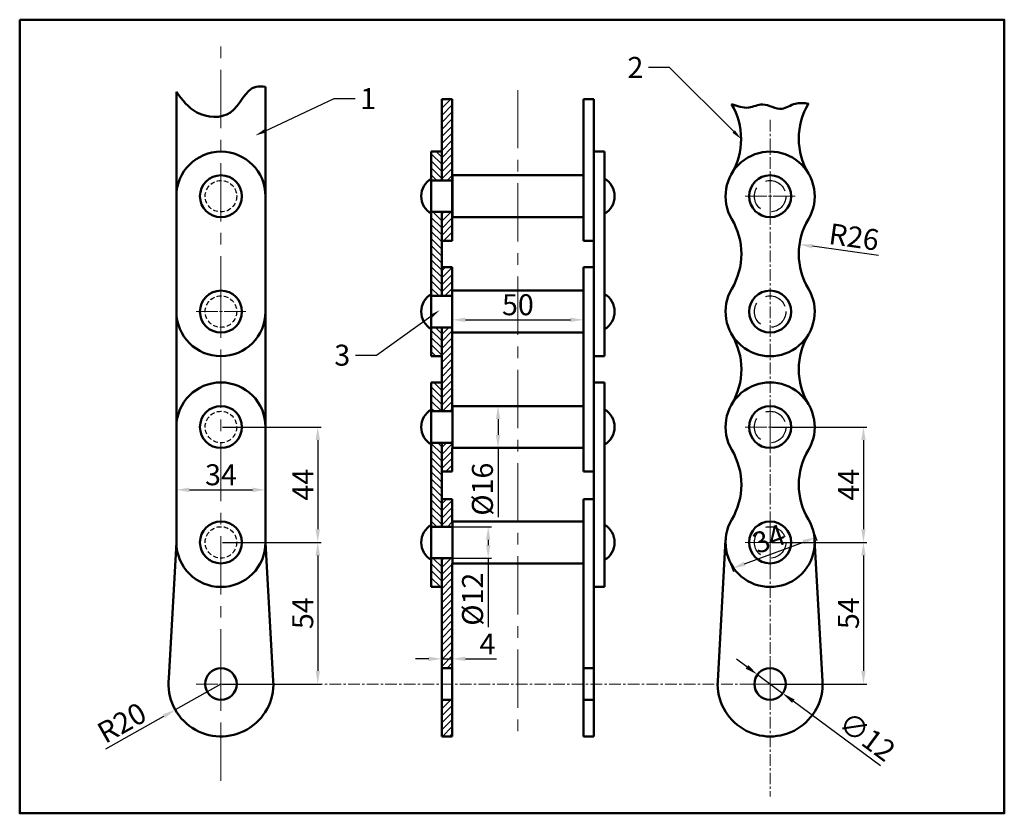
# Model space of a CAD drawing. Units: millimetres. Extents: x 359 to 734, y 213 to 516.
import ezdxf
from ezdxf import colors
from ezdxf.entities.mleader import LeaderData, LeaderLine
from ezdxf.math import Vec2, Vec3

# ---------------------------------------------------------------- set-up
doc = ezdxf.new("R2010")
doc.units = ezdxf.units.MM
doc.header["$LTSCALE"] = 0.7
doc.linetypes.add('CENTER', pattern=[50.8, 31.75, -6.35, 6.35, -6.35])
doc.linetypes.add('DASHED', pattern=[19.05, 12.7, -6.35])
for name, color, linetype, lineweight in [('M-CNTR', 1, 'CENTER', 18), ('M-DIMS', 2, 'Continuous', 25), ('M-HATC', 8, 'Continuous', 18), ('M-HIDN', 6, 'DASHED', 25), ('M-OUTL', 7, 'Continuous', 50), ('M-TTLB', 7, 'Continuous', 50)]:
    doc.layers.add(name, color=color, linetype=linetype, lineweight=lineweight)
doc.styles.get("Standard").update_dxf_attribs({"font": 'arial.ttf'})
doc.dimstyles.new('ISO-25', dxfattribs={"dimtxt": 8, "dimasz": 5, "dimexe": 1.25, "dimexo": 0.625, "dimtad": 1, "dimdec": 0, "dimtxsty": 'Standard', "dimcen": 2.5, "dimadec": 0, "dimazin": 0, "dimtfac": 1, "dimtdec": 0, "dimtmove": 0, "dimatfit": 3, "dimfxl": 1, "dimarcsym": 0})

# ---------------------------------------------------------------- blocks, each defined once
blk = doc.blocks.new('*U1')
at = {"layer": 'M-CNTR', "color": 0, "transparency": 16777216}
for p, q in [((0, 1.2), (0, 9.5)), ((-9.5, 0), (-1.2, 0)), ((1.2, 0), (9.5, 0)), ((0, -9.5), (0, -1.2))]:
    blk.add_line(p, q, dxfattribs=at)
at = {"layer": 'M-CNTR', "color": 0, "linetype": 'Continuous', "transparency": 16777216}
for p, q in [((-0.6, 0), (0.6, 0)), ((0, -0.6), (0, 0.6))]:
    blk.add_line(p, q, dxfattribs=at)
blk = doc.blocks.new('*U2')
at = {"layer": 'M-CNTR', "color": 0, "transparency": 16777216}
for p, q in [((0, 1.2), (0, 9.5)), ((-9.5, 0), (-1.2, 0)), ((1.2, 0), (9.5, 0)), ((0, -9.5), (0, -1.2))]:
    blk.add_line(p, q, dxfattribs=at)
at = {"layer": 'M-CNTR', "color": 0, "linetype": 'Continuous', "transparency": 16777216}
for p, q in [((-0.6, 0), (0.6, 0)), ((0, -0.6), (0, 0.6))]:
    blk.add_line(p, q, dxfattribs=at)
blk = doc.blocks.new('*U3')
at = {"layer": 'M-CNTR', "color": 0, "transparency": 16777216}
for p, q in [((0, 1.2), (0, 9.5)), ((-9.5, 0), (-1.2, 0)), ((1.2, 0), (9.5, 0)), ((0, -9.5), (0, -1.2))]:
    blk.add_line(p, q, dxfattribs=at)
at = {"layer": 'M-CNTR', "color": 0, "linetype": 'Continuous', "transparency": 16777216}
for p, q in [((-0.6, 0), (0.6, 0)), ((0, -0.6), (0, 0.6))]:
    blk.add_line(p, q, dxfattribs=at)
blk = doc.blocks.new('*U4')
at = {"layer": 'M-CNTR', "color": 0, "transparency": 16777216}
for p, q in [((0, 1.2), (0, 9.5)), ((-9.5, 0), (-1.2, 0)), ((1.2, 0), (9.5, 0)), ((0, -9.5), (0, -1.2))]:
    blk.add_line(p, q, dxfattribs=at)
at = {"layer": 'M-CNTR', "color": 0, "linetype": 'Continuous', "transparency": 16777216}
for p, q in [((-0.6, 0), (0.6, 0)), ((0, -0.6), (0, 0.6))]:
    blk.add_line(p, q, dxfattribs=at)
blk = doc.blocks.new('*U5')
at = {"layer": 'M-CNTR', "color": 0, "transparency": 16777216}
for p, q in [((0, 1.2), (0, 9.5)), ((-9.5, 0), (-1.2, 0)), ((1.2, 0), (9.5, 0)), ((0, -9.5), (0, -1.2))]:
    blk.add_line(p, q, dxfattribs=at)
at = {"layer": 'M-CNTR', "color": 0, "linetype": 'Continuous', "transparency": 16777216}
for p, q in [((-0.6, 0), (0.6, 0)), ((0, -0.6), (0, 0.6))]:
    blk.add_line(p, q, dxfattribs=at)
blk = doc.blocks.new('*U6')
at = {"layer": 'M-CNTR', "color": 0, "transparency": 16777216}
for p, q in [((0, 1.2), (0, 9.5)), ((-9.5, 0), (-1.2, 0)), ((1.2, 0), (9.5, 0)), ((0, -9.5), (0, -1.2))]:
    blk.add_line(p, q, dxfattribs=at)
at = {"layer": 'M-CNTR', "color": 0, "linetype": 'Continuous', "transparency": 16777216}
for p, q in [((-0.6, 0), (0.6, 0)), ((0, -0.6), (0, 0.6))]:
    blk.add_line(p, q, dxfattribs=at)
blk = doc.blocks.new('*U7')
at = {"layer": 'M-CNTR', "color": 0, "transparency": 16777216}
blk.add_line((0, 18), (0, -229.67), dxfattribs=at)
blk = doc.blocks.new('*U8')
at = {"layer": 'M-CNTR', "color": 0, "transparency": 16777216}
blk.add_line((0, -156.93), (0, 123.49), dxfattribs=at)
blk = doc.blocks.new('*D9')
at = {"layer": 'Defpoints', "color": 0, "ltscale": 0.7, "transparency": 16777216}
for p in [(418.66, 336.41), (452.66, 336.64), (452.66, 336.41)]:
    blk.add_point(p, dxfattribs=at)
at = {"layer": 'M-DIMS', "color": 0, "lineweight": -2, "ltscale": 0.7, "transparency": 16777216}
for p, q in [((418.66, 337.04), (418.66, 337.89)), ((452.66, 337.04), (452.66, 337.89)), ((423.66, 336.64), (447.66, 336.64))]:
    blk.add_line(p, q, dxfattribs=at)
at = {"layer": 'M-DIMS', "color": 0, "ltscale": 0.7, "transparency": 16777216}
for points in [[(423.66, 337.48), (423.66, 335.81), (418.66, 336.64)], [(447.66, 337.48), (447.66, 335.81), (452.66, 336.64)]]:
    blk.add_solid(points, dxfattribs=at)
at = {"layer": 'M-DIMS', "color": 0, "ltscale": 0.7, "transparency": 16777216, "insert": (435.66, 341.35), "char_height": 8, "attachment_point": 5}
blk.add_mtext('34', dxfattribs=at)
blk = doc.blocks.new('*D10')
at = {"layer": 'Defpoints', "color": 0, "ltscale": 0.7, "transparency": 16777216}
for p in [(435.66, 360.6), (435.66, 316.6), (472.57, 316.6)]:
    blk.add_point(p, dxfattribs=at)
at = {"layer": 'M-DIMS', "color": 0, "lineweight": -2, "ltscale": 0.7, "transparency": 16777216}
for p, q in [((436.28, 360.6), (473.82, 360.6)), ((472.57, 355.6), (472.57, 321.6)), ((436.28, 316.6), (473.82, 316.6))]:
    blk.add_line(p, q, dxfattribs=at)
at = {"layer": 'M-DIMS', "color": 0, "ltscale": 0.7, "transparency": 16777216}
for points in [[(471.73, 355.6), (473.4, 355.6), (472.57, 360.6)], [(471.73, 321.6), (473.4, 321.6), (472.57, 316.6)]]:
    blk.add_solid(points, dxfattribs=at)
at = {"layer": 'M-DIMS', "color": 0, "ltscale": 0.7, "transparency": 16777216, "insert": (467.94, 338.6), "char_height": 8, "attachment_point": 5, "rotation": 90}
blk.add_mtext('44', dxfattribs=at)
blk = doc.blocks.new('*D11')
at = {"layer": 'Defpoints', "color": 0, "ltscale": 0.7, "transparency": 16777216}
for p in [(463.42, 316.6), (435.66, 262.6), (472.57, 262.6)]:
    blk.add_point(p, dxfattribs=at)
at = {"layer": 'M-DIMS', "color": 0, "lineweight": -2, "ltscale": 0.7, "transparency": 16777216}
for p, q in [((464.04, 316.6), (473.82, 316.6)), ((472.57, 311.6), (472.57, 267.6)), ((436.28, 262.6), (473.82, 262.6))]:
    blk.add_line(p, q, dxfattribs=at)
at = {"layer": 'M-DIMS', "color": 0, "ltscale": 0.7, "transparency": 16777216}
for points in [[(471.73, 311.6), (473.4, 311.6), (472.57, 316.6)], [(471.73, 267.6), (473.4, 267.6), (472.57, 262.6)]]:
    blk.add_solid(points, dxfattribs=at)
at = {"layer": 'M-DIMS', "color": 0, "ltscale": 0.7, "transparency": 16777216, "insert": (467.87, 289.6), "char_height": 8, "attachment_point": 5, "rotation": 90}
blk.add_mtext('54', dxfattribs=at)
blk = doc.blocks.new('*D12')
at = {"layer": 'Defpoints', "color": 0, "ltscale": 0.7, "transparency": 16777216}
for p in [(523.86, 404.6), (573.86, 404.6), (573.86, 401.48)]:
    blk.add_point(p, dxfattribs=at)
at = {"layer": 'M-DIMS', "color": 0, "lineweight": -2, "ltscale": 0.7, "transparency": 16777216}
for p, q in [((523.86, 403.97), (523.86, 400.23)), ((573.86, 403.97), (573.86, 400.23)), ((528.86, 401.48), (568.86, 401.48))]:
    blk.add_line(p, q, dxfattribs=at)
at = {"layer": 'M-DIMS', "color": 0, "ltscale": 0.7, "transparency": 16777216}
for points in [[(528.86, 402.31), (528.86, 400.65), (523.86, 401.48)], [(568.86, 402.31), (568.86, 400.65), (573.86, 401.48)]]:
    blk.add_solid(points, dxfattribs=at)
at = {"layer": 'M-DIMS', "color": 0, "ltscale": 0.7, "transparency": 16777216, "insert": (548.86, 406.19), "char_height": 8, "attachment_point": 5}
blk.add_mtext('50', dxfattribs=at)
blk = doc.blocks.new('*D13')
at = {"layer": 'Defpoints', "color": 0, "ltscale": 0.7, "transparency": 16777216}
for p in [(541.3, 368.6), (541.3, 352.6), (541.3, 352.6)]:
    blk.add_point(p, dxfattribs=at)
at = {"layer": 'M-DIMS', "color": 0, "lineweight": -2, "ltscale": 0.7, "transparency": 16777216}
for p, q in [((541.93, 368.6), (542.55, 368.6)), ((541.3, 363.6), (541.3, 357.6)), ((541.3, 352.6), (541.3, 326.19)), ((541.93, 352.6), (542.55, 352.6))]:
    blk.add_line(p, q, dxfattribs=at)
at = {"layer": 'M-DIMS', "color": 0, "ltscale": 0.7, "transparency": 16777216}
for points in [[(540.47, 363.6), (542.13, 363.6), (541.3, 368.6)], [(540.47, 357.6), (542.13, 357.6), (541.3, 352.6)]]:
    blk.add_solid(points, dxfattribs=at)
at = {"layer": 'M-DIMS', "color": 0, "ltscale": 0.7, "transparency": 16777216, "insert": (536.37, 336.89), "char_height": 8, "attachment_point": 5, "rotation": 90}
blk.add_mtext('%%C16', dxfattribs=at)
blk = doc.blocks.new('*D14')
at = {"layer": 'Defpoints', "color": 0, "ltscale": 0.7, "transparency": 16777216}
for p in [(523.86, 322.6), (523.86, 310.6), (537.54, 310.6)]:
    blk.add_point(p, dxfattribs=at)
at = {"layer": 'M-DIMS', "color": 0, "lineweight": -2, "ltscale": 0.7, "transparency": 16777216}
for p, q in [((524.49, 322.6), (538.79, 322.6)), ((537.54, 317.6), (537.54, 315.6)), ((524.49, 310.6), (538.79, 310.6)), ((537.54, 310.6), (537.54, 284.26))]:
    blk.add_line(p, q, dxfattribs=at)
at = {"layer": 'M-DIMS', "color": 0, "ltscale": 0.7, "transparency": 16777216}
for points in [[(536.7, 317.6), (538.37, 317.6), (537.54, 322.6)], [(536.7, 315.6), (538.37, 315.6), (537.54, 310.6)]]:
    blk.add_solid(points, dxfattribs=at)
at = {"layer": 'M-DIMS', "color": 0, "ltscale": 0.7, "transparency": 16777216, "insert": (532.6, 294.93), "char_height": 8, "attachment_point": 5, "rotation": 90}
blk.add_mtext('%%C12', dxfattribs=at)
blk = doc.blocks.new('*D15')
at = {"layer": 'Defpoints', "color": 0, "ltscale": 0.7, "transparency": 16777216}
for p in [(645.01, 360.6), (645.01, 316.6), (680.58, 316.6)]:
    blk.add_point(p, dxfattribs=at)
at = {"layer": 'M-DIMS', "color": 0, "lineweight": -2, "ltscale": 0.7, "transparency": 16777216}
for p, q in [((645.63, 360.6), (681.83, 360.6)), ((680.58, 355.6), (680.58, 321.6)), ((645.63, 316.6), (681.83, 316.6))]:
    blk.add_line(p, q, dxfattribs=at)
at = {"layer": 'M-DIMS', "color": 0, "ltscale": 0.7, "transparency": 16777216}
for points in [[(679.75, 355.6), (681.41, 355.6), (680.58, 360.6)], [(679.75, 321.6), (681.41, 321.6), (680.58, 316.6)]]:
    blk.add_solid(points, dxfattribs=at)
at = {"layer": 'M-DIMS', "color": 0, "ltscale": 0.7, "transparency": 16777216, "insert": (675.95, 338.6), "char_height": 8, "attachment_point": 5, "rotation": 90}
blk.add_mtext('44', dxfattribs=at)
blk = doc.blocks.new('*D16')
at = {"layer": 'Defpoints', "color": 0, "ltscale": 0.7, "transparency": 16777216}
for p in [(645.01, 316.6), (645.01, 262.6), (680.58, 262.6)]:
    blk.add_point(p, dxfattribs=at)
at = {"layer": 'M-DIMS', "color": 0, "lineweight": -2, "ltscale": 0.7, "transparency": 16777216}
for p, q in [((645.63, 316.6), (681.83, 316.6)), ((680.58, 311.6), (680.58, 267.6)), ((645.63, 262.6), (681.83, 262.6))]:
    blk.add_line(p, q, dxfattribs=at)
at = {"layer": 'M-DIMS', "color": 0, "ltscale": 0.7, "transparency": 16777216}
for points in [[(679.75, 311.6), (681.41, 311.6), (680.58, 316.6)], [(679.75, 267.6), (681.41, 267.6), (680.58, 262.6)]]:
    blk.add_solid(points, dxfattribs=at)
at = {"layer": 'M-DIMS', "color": 0, "ltscale": 0.7, "transparency": 16777216, "insert": (675.89, 289.6), "char_height": 8, "attachment_point": 5, "rotation": 90}
blk.add_mtext('54', dxfattribs=at)
blk = doc.blocks.new('*D17')
at = {"layer": 'Defpoints', "color": 0, "ltscale": 0.7, "transparency": 16777216}
for p in [(661.29, 321.47), (662.4, 318.5), (629.49, 309.66)]:
    blk.add_point(p, dxfattribs=at)
at = {"layer": 'M-DIMS', "color": 0, "lineweight": -2, "ltscale": 0.7, "transparency": 16777216}
for p, q in [((661.51, 320.88), (662.83, 317.32)), ((635.28, 308.42), (657.71, 316.75)), ((629.71, 309.07), (631.03, 305.51))]:
    blk.add_line(p, q, dxfattribs=at)
at = {"layer": 'M-DIMS', "color": 0, "ltscale": 0.7, "transparency": 16777216}
for points in [[(657.42, 317.54), (658, 315.97), (662.4, 318.5)], [(634.99, 309.2), (635.57, 307.64), (630.59, 306.68)]]:
    blk.add_solid(points, dxfattribs=at)
at = {"layer": 'M-DIMS', "color": 0, "ltscale": 0.7, "transparency": 16777216, "insert": (644.86, 317.01), "char_height": 8, "attachment_point": 5, "rotation": 20.3752}
blk.add_mtext('34', dxfattribs=at)
blk = doc.blocks.new('*D18')
at = {"layer": 'Defpoints', "color": 0, "ltscale": 0.7, "transparency": 16777216}
for p in [(656.21, 430.22), (681.95, 426.6)]:
    blk.add_point(p, dxfattribs=at)
at = {"layer": 'M-DIMS', "color": 0, "lineweight": -2, "ltscale": 0.7, "transparency": 16777216}
blk.add_line((686.27, 425.99), (661.16, 429.52), dxfattribs=at)
at = {"layer": 'M-DIMS', "color": 0, "ltscale": 0.7, "transparency": 16777216}
blk.add_solid([(661.28, 430.35), (661.04, 428.7), (656.21, 430.22)], dxfattribs=at)
at = {"layer": 'M-DIMS', "color": 0, "ltscale": 0.7, "transparency": 16777216, "insert": (676.85, 432.07), "char_height": 8, "attachment_point": 5, "rotation": 351.9866}
blk.add_mtext('R26', dxfattribs=at)
blk = doc.blocks.new('*D19')
at = {"layer": 'Defpoints', "color": 0, "ltscale": 0.7, "transparency": 16777216}
for p in [(435.66, 262.6), (418.24, 252.76)]:
    blk.add_point(p, dxfattribs=at)
at = {"layer": 'M-DIMS', "color": 0, "lineweight": -2, "ltscale": 0.7, "transparency": 16777216}
for p, q in [((435.66, 262.6), (418.24, 252.76)), ((391.83, 237.84), (413.89, 250.3))]:
    blk.add_line(p, q, dxfattribs=at)
at = {"layer": 'M-DIMS', "color": 0, "ltscale": 0.7, "transparency": 16777216}
blk.add_solid([(413.48, 251.03), (414.3, 249.58), (418.24, 252.76)], dxfattribs=at)
at = {"layer": 'M-DIMS', "color": 0, "ltscale": 0.7, "transparency": 16777216, "insert": (398.37, 246.94), "char_height": 8, "attachment_point": 5, "rotation": 29.4552}
blk.add_mtext('R20', dxfattribs=at)
blk = doc.blocks.new('*D20')
at = {"layer": 'Defpoints', "color": 0, "ltscale": 0.7, "transparency": 16777216}
for p in [(640.19, 266.17), (649.83, 259.02)]:
    blk.add_point(p, dxfattribs=at)
at = {"layer": 'M-DIMS', "color": 0, "lineweight": -2, "ltscale": 0.7, "transparency": 16777216}
for p, q in [((636.17, 269.15), (632.15, 272.12)), ((640.19, 266.17), (649.83, 259.02)), ((687.03, 231.46), (653.85, 256.05))]:
    blk.add_line(p, q, dxfattribs=at)
at = {"layer": 'M-DIMS', "color": 0, "ltscale": 0.7, "transparency": 16777216}
for points in [[(636.67, 269.82), (635.67, 268.48), (640.19, 266.17)], [(654.34, 256.72), (653.35, 255.38), (649.83, 259.02)]]:
    blk.add_solid(points, dxfattribs=at)
at = {"layer": 'M-DIMS', "color": 0, "ltscale": 0.7, "transparency": 16777216, "insert": (681.4, 241.77), "char_height": 8, "attachment_point": 5, "rotation": 323.4618}
blk.add_mtext('∅12', dxfattribs=at)
blk = doc.blocks.new('*D21')
at = {"layer": 'Defpoints', "color": 0, "ltscale": 0.7, "transparency": 16777216}
for p in [(519.86, 271.1), (523.86, 272.19), (523.86, 271.1)]:
    blk.add_point(p, dxfattribs=at)
at = {"layer": 'M-DIMS', "color": 0, "lineweight": -2, "ltscale": 0.7, "transparency": 16777216}
for p, q in [((514.86, 272.19), (509.86, 272.19)), ((519.86, 271.72), (519.86, 273.44)), ((519.86, 272.19), (523.86, 272.19)), ((523.86, 271.72), (523.86, 273.44)), ((528.86, 272.19), (540.64, 272.19))]:
    blk.add_line(p, q, dxfattribs=at)
at = {"layer": 'M-DIMS', "color": 0, "ltscale": 0.7, "transparency": 16777216}
for points in [[(514.86, 273.03), (514.86, 271.36), (519.86, 272.19)], [(528.86, 273.03), (528.86, 271.36), (523.86, 272.19)]]:
    blk.add_solid(points, dxfattribs=at)
at = {"layer": 'M-DIMS', "color": 0, "ltscale": 0.7, "transparency": 16777216, "insert": (537.25, 276.82), "char_height": 8, "attachment_point": 5}
blk.add_mtext('4', dxfattribs=at)
blk = doc.blocks.new('CHAIN-PIN')
at = {"ltscale": 0.2}
for p, q in [((11.84, 16), (61.84, 16)), ((11.84, 16), (11.84, 0)), ((61.84, 16), (61.84, 0)), ((61.84, 0), (11.84, 0))]:
    blk.add_line(p, q, dxfattribs=at)
for centre, start, end in [((7.77, 8), 120.36, 239.64), ((65.92, 8), 300.36, 59.64)]:
    blk.add_arc(centre, 7.77, start, end, dxfattribs=at)

msp = doc.modelspace()

# ---------------------------------------------------------------- hatches: boundary and pattern name
at = {"layer": 'M-HATC', "ltscale": 0.2}
h = msp.add_hatch(dxfattribs=at)
h.set_pattern_fill('ANSI31', color=256, scale=0.6)
h.paths.add_polyline_path([(523.86, 485.6), (519.86, 485.6), (519.86, 465.6), (519.86, 454.6), (523.86, 454.6), (523.86, 456.6)])
h.paths.add_polyline_path([(523.86, 442.6), (519.86, 442.6), (519.86, 431.6), (523.86, 431.6)])
h.paths.add_polyline_path([(523.86, 421.6), (519.86, 421.6), (519.86, 410.6), (523.86, 410.6)])
h.paths.add_polyline_path([(523.86, 396.6), (523.86, 398.6), (519.86, 398.6), (519.86, 387.6), (519.86, 377.6), (519.86, 366.6), (523.86, 366.6)])
h.paths.add_polyline_path([(523.86, 352.6), (523.86, 354.6), (519.86, 354.6), (519.86, 343.6), (523.86, 343.6)])
h.paths.add_polyline_path([(523.86, 333.1), (519.86, 333.1), (519.86, 322.6), (523.86, 322.6), (523.86, 324.6)])
h.paths.add_polyline_path([(523.86, 308.6), (523.86, 310.6), (519.86, 310.6), (519.86, 299.6), (519.86, 268.6), (523.86, 268.6)])
h.paths.add_polyline_path([(523.86, 256.6), (519.86, 256.6), (519.86, 242.6), (523.86, 242.6)])
h = msp.add_hatch(dxfattribs=at)
h.set_pattern_fill('ANSI31', color=256, scale=0.6, angle=90)
h.paths.add_polyline_path([(519.86, 310.6), (515.86, 310.6), (515.86, 299.6), (519.86, 299.6)])
h.paths.add_polyline_path([(519.86, 343.6), (519.86, 354.6), (515.86, 354.6), (515.86, 322.6), (519.86, 322.6)])
h.paths.add_polyline_path([(519.86, 377.6), (515.86, 377.6), (515.86, 366.6), (519.86, 366.6)])
h.paths.add_polyline_path([(519.86, 398.6), (515.86, 398.6), (515.86, 387.6), (519.86, 387.6)])
h.paths.add_polyline_path([(519.86, 431.6), (519.86, 442.6), (515.86, 442.6), (515.86, 431.6), (515.86, 410.6), (519.86, 410.6)])
h.paths.add_polyline_path([(519.86, 465.6), (515.86, 465.6), (515.86, 454.6), (519.86, 454.6)])

# ---------------------------------------------------------------- linework, layer by layer
at = {"layer": 'M-CNTR', "ltscale": 0.2}
for p, q in [((645.01, 477.71), (645.01, 219.69)), ((455.66, 262.6), (435.66, 262.6)), ((645.01, 262.6), (455.66, 262.6))]:
    msp.add_line(p, q, dxfattribs=at)
at = {"layer": 'M-HIDN', "ltscale": 0.2}
for centre in [(435.66, 448.6), (435.66, 404.6), (435.66, 360.6), (435.66, 316.6)]:
    msp.add_circle(centre, 6, dxfattribs=at)
at = {"layer": 'M-HIDN'}
for centre in [(645.01, 448.6), (645.01, 404.6), (645.01, 360.6), (645.01, 316.6)]:
    msp.add_circle(centre, 6, dxfattribs=at)
at = {"layer": 'M-OUTL', "ltscale": 0.2}
for p, q in [((418.66, 448.6), (418.66, 488.4)), ((452.66, 448.6), (452.66, 490.34)), ((519.86, 465.6), (519.86, 485.6)), ((519.86, 485.6), (523.86, 485.6)), ((523.86, 485.6), (523.86, 456.6)), ((577.86, 485.6), (573.86, 485.6)), ((573.86, 485.6), (573.86, 456.6)), ((577.86, 465.6), (577.86, 485.6)), ((515.86, 431.6), (515.86, 465.6)), ((519.86, 465.6), (515.86, 465.6)), ((519.86, 454.6), (519.86, 465.6)), ((577.86, 431.6), (577.86, 465.6)), ((577.86, 454.6), (577.86, 465.6)), ((577.86, 465.6), (581.86, 465.6)), ((581.86, 431.6), (581.86, 465.6)), ((515.86, 454.6), (523.86, 454.6)), ((523.86, 431.6), (523.86, 456.6)), ((573.86, 431.6), (573.86, 456.6)), ((418.66, 316.6), (418.66, 448.6)), ((452.66, 448.6), (452.66, 316.6)), ((515.86, 442.6), (523.86, 442.6)), ((519.86, 431.6), (519.86, 442.6)), ((515.86, 431.6), (515.86, 410.6)), ((523.86, 431.6), (519.86, 431.6)), ((519.86, 410.6), (519.86, 431.6)), ((573.86, 431.6), (577.86, 431.6)), ((577.86, 410.6), (577.86, 431.6)), ((581.86, 431.6), (581.86, 410.6)), ((519.86, 421.6), (523.86, 421.6)), ((523.86, 421.6), (523.86, 410.6)), ((577.86, 421.6), (573.86, 421.6)), ((573.86, 421.6), (573.86, 410.6)), ((577.86, 387.6), (577.86, 421.6)), ((523.86, 410.6), (515.86, 410.6)), ((515.86, 410.6), (515.86, 387.6)), ((573.86, 412.6), (573.86, 396.6)), ((581.86, 410.6), (581.86, 387.6)), ((515.86, 398.6), (523.86, 398.6)), ((519.86, 387.6), (519.86, 398.6)), ((523.86, 396.6), (523.86, 366.6)), ((573.86, 396.6), (573.86, 366.6)), ((515.86, 387.6), (519.86, 387.6)), ((519.86, 387.6), (519.86, 377.6)), ((581.86, 387.6), (577.86, 387.6)), ((577.86, 387.6), (577.86, 377.6)), ((515.86, 377.6), (519.86, 377.6)), ((515.86, 366.6), (515.86, 377.6)), ((519.86, 377.6), (519.86, 366.6)), ((581.86, 377.6), (577.86, 377.6)), ((577.86, 377.6), (577.86, 360.6)), ((581.86, 366.6), (581.86, 377.6)), ((573.86, 368.6), (573.86, 352.6)), ((523.86, 366.6), (515.86, 366.6)), ((515.86, 366.6), (515.86, 354.6)), ((581.86, 366.6), (581.86, 354.6)), ((577.86, 343.6), (577.86, 360.6)), ((515.86, 354.6), (523.86, 354.6)), ((515.86, 354.6), (515.86, 322.6)), ((519.86, 343.6), (519.86, 354.6)), ((581.86, 354.6), (581.86, 322.6)), ((523.86, 352.6), (523.86, 343.6)), ((573.86, 352.6), (573.86, 343.6)), ((523.86, 343.6), (519.86, 343.6)), ((519.86, 343.6), (519.86, 322.6)), ((573.86, 343.6), (577.86, 343.6)), ((577.86, 343.6), (577.86, 299.6)), ((519.86, 333.1), (523.86, 333.1)), ((523.86, 333.1), (523.86, 324.6)), ((577.86, 333.1), (573.86, 333.1)), ((573.86, 333.1), (573.86, 324.6)), ((523.86, 322.6), (515.86, 322.6)), ((515.86, 322.6), (515.86, 310.6)), ((581.86, 322.6), (581.86, 310.6)), ((418.66, 316.6), (415.78, 264.81)), ((452.66, 316.6), (455.63, 263.72)), ((628.03, 317.54), (625.04, 263.71)), ((661.98, 317.54), (664.98, 263.71)), ((515.86, 310.6), (523.86, 310.6)), ((515.86, 310.6), (515.86, 299.6)), ((519.86, 299.6), (519.86, 310.6)), ((523.86, 308.6), (523.86, 242.6)), ((573.86, 308.6), (573.86, 242.6)), ((577.86, 299.6), (577.86, 310.6)), ((581.86, 310.6), (581.86, 299.6)), ((515.86, 299.6), (519.86, 299.6)), ((519.86, 242.6), (519.86, 299.6)), ((581.86, 299.6), (577.86, 299.6)), ((577.86, 242.6), (577.86, 299.6)), ((519.86, 268.6), (523.86, 268.6)), ((577.86, 268.6), (573.86, 268.6)), ((519.86, 256.6), (523.86, 256.6)), ((577.86, 256.6), (573.86, 256.6)), ((523.86, 242.6), (519.86, 242.6)), ((577.86, 242.6), (573.86, 242.6))]:
    msp.add_line(p, q, dxfattribs=at)
for centre, radius in [((435.66, 448.6), 8), ((435.66, 404.6), 8), ((435.66, 360.6), 8), ((435.66, 316.6), 8), ((435.66, 262.6), 6), ((645.01, 262.6), 6)]:
    msp.add_circle(centre, radius, dxfattribs=at)
at = {"layer": 'M-OUTL'}
for centre in [(645.01, 448.6), (645.01, 404.6), (645.01, 360.6), (645.01, 316.6)]:
    msp.add_circle(centre, 8, dxfattribs=at)
for centre, radius, start, end in [((607.96, 470.42), 26, 329.2277, 30.7723), ((681.95, 470.6), 26, 149.2277, 210.7723), ((645.01, 448.6), 17, 329.2277, 210.7723), ((608.06, 426.6), 26, 329.2277, 30.7723), ((681.95, 426.6), 26, 149.2277, 210.7723), ((645.01, 404.6), 17, 149.2277, 30.7723), ((645.01, 360.6), 17, 329.2277, 210.7723), ((608.06, 338.6), 26, 329.2277, 30.7723), ((681.95, 338.6), 26, 149.2277, 210.7723), ((645.01, 316.6), 17, 149.2277, 30.7723)]:
    msp.add_arc(centre, radius, start, end, dxfattribs=at)
at = {"layer": 'M-OUTL', "ltscale": 0.2}
for centre, radius, start, end in [((435.66, 448.6), 17, 0, 180), ((435.66, 448.6), 17, 0, 180), ((435.66, 404.6), 17, 180, 0), ((435.66, 404.6), 17, 180, 0), ((608.06, 382.6), 26, 329.2277, 30.7723), ((681.95, 382.6), 26, 149.2277, 210.7723), ((435.66, 360.6), 17, 0, 180), ((435.66, 360.6), 17, 0, 180), ((435.66, 316.6), 17, 180, 0), ((435.66, 316.6), 17, 180, 0), ((435.66, 262.6), 20, 173.6403, 3.2131), ((645.01, 262.6), 20, 176.8153, 3.1847)]:
    msp.add_arc(centre, radius, start, end, dxfattribs=at)
for points, knots in [([(418.66, 488.4), (420.9, 485.37), (425.72, 478.87), (441.5, 477.59), (445.31, 491.04), (451.4, 490.46), (452.66, 490.34)], [0, 0, 0, 0, 11.086595, 23.847692, 37.683021, 41.299462, 41.299462, 41.299462, 41.299462]), ([(630.3, 483.73), (632.49, 482.94), (636.47, 481.51), (642.8, 484.87), (648.91, 480.41), (654.3, 484.57), (657.88, 484.1), (659.6, 483.88)], [0, 0, 0, 0, 6.674591, 12.150347, 19.536339, 25.002981, 30.07651, 30.07651, 30.07651, 30.07651])]:
    msp.add_open_spline(points, degree=3, knots=knots, dxfattribs=at)
at = {"layer": 'M-TTLB', "ltscale": 0.7}
msp.add_lwpolyline([(358.94, 515.93), (734.28, 515.93), (734.28, 213.29), (358.94, 213.29)], close=True, dxfattribs=at)

# ---------------------------------------------------------------- block references
at = {"layer": 'M-CNTR'}
for name, p in [('*U8', (435.66, 382.6)), ('*U7', (548.86, 471.1)), ('*U6', (645.01, 448.6)), ('*U1', (435.66, 404.6)), ('*U5', (645.01, 360.6)), ('*U4', (645.01, 316.6)), ('*U2', (435.66, 262.6)), ('*U3', (645.01, 262.6))]:
    msp.add_blockref(name, p, dxfattribs=at)
at = {"layer": 'M-OUTL', "rotation": 180}
for p in [(585.71, 456.6), (585.71, 368.6), (585.71, 324.6)]:
    msp.add_blockref('CHAIN-PIN', p, dxfattribs=at)
at = {"layer": 'M-OUTL'}
msp.add_blockref('CHAIN-PIN', (512.02, 396.6), dxfattribs=at)

# ---------------------------------------------------------------- dimensions: what is measured, and where the dimension line sits
at = {"layer": 'M-DIMS', "ltscale": 0.7}
dim = msp.add_radius_dim(center=(681.95, 426.6), mpoint=(656.21, 430.22), dimstyle='ISO-25', override={"dimclrd": 0, "dimclre": 0, "dimclrt": 0}, dxfattribs=at)
dim.commit()
dim.dimension.update_dxf_attribs({"geometry": '*D18', "text_midpoint": (676.19, 427.41), "dimtype": 164})
for base, p1, p2, picture, middle in [((573.86, 401.48), (523.86, 404.6), (573.86, 404.6), '*D12', (548.86, 406.19)), ((452.66, 336.64), (418.66, 336.41), (452.66, 336.41), '*D9', (435.66, 341.35)), ((523.86, 272.19), (519.86, 271.1), (523.86, 271.1), '*D21', (537.25, 276.82))]:
    dim = msp.add_linear_dim(base=base, p1=p1, p2=p2, dimstyle='ISO-25', override={"dimclrd": 0, "dimclre": 0, "dimclrt": 0}, dxfattribs=at)
    dim.commit()
    dim.dimension.update_dxf_attribs({"geometry": picture, "text_midpoint": middle})
for base, p1, p2, text, picture, middle in [((541.3, 352.6), (541.3, 368.6), (541.3, 352.6), '%%C<>', '*D13', (536.37, 336.89)), ((537.54, 310.6), (523.86, 322.6), (523.86, 310.6), '%%C12', '*D14', (532.6, 294.93))]:
    dim = msp.add_linear_dim(base=base, p1=p1, p2=p2, angle=90, text=text, dimstyle='ISO-25', override={"dimclrd": 0, "dimclre": 0, "dimclrt": 0}, dxfattribs=at)
    dim.commit()
    dim.dimension.update_dxf_attribs({"geometry": picture, "text_midpoint": middle})
for base, p1, p2, picture, middle in [((472.57, 316.6), (435.66, 360.6), (435.66, 316.6), '*D10', (467.94, 338.6)), ((680.58, 316.6), (645.01, 360.6), (645.01, 316.6), '*D15', (675.95, 338.6)), ((472.57, 262.6), (463.42, 316.6), (435.66, 262.6), '*D11', (467.87, 289.6)), ((680.58, 262.6), (645.01, 316.6), (645.01, 262.6), '*D16', (675.89, 289.6))]:
    dim = msp.add_linear_dim(base=base, p1=p1, p2=p2, angle=90, dimstyle='ISO-25', override={"dimclrd": 0, "dimclre": 0, "dimclrt": 0}, dxfattribs=at)
    dim.commit()
    dim.dimension.update_dxf_attribs({"geometry": picture, "text_midpoint": middle})
dim = msp.add_aligned_dim(p1=(629.49, 309.66), p2=(661.29, 321.47), distance=-3.17, dimstyle='ISO-25', override={"dimclrd": 0, "dimclre": 0, "dimclrt": 0}, dxfattribs=at)
dim.commit()
dim.dimension.update_dxf_attribs({"geometry": '*D17', "text_midpoint": (644.86, 317.01)})
dim = msp.add_diameter_dim_2p(p1=(640.19, 266.17), p2=(649.83, 259.02), dimstyle='ISO-25', override={"dimclrd": 0, "dimclre": 0, "dimclrt": 0}, dxfattribs=at)
dim.commit()
dim.dimension.update_dxf_attribs({"geometry": '*D20', "text_midpoint": (678.46, 237.81), "dimtype": 163})
dim = msp.add_radius_dim(center=(435.66, 262.6), mpoint=(418.24, 252.76), dimstyle='ISO-25', override={"dimclrd": 0, "dimclre": 0, "dimclrt": 0}, dxfattribs=at)
dim.commit()
dim.dimension.update_dxf_attribs({"geometry": '*D19', "text_midpoint": (398.37, 246.94)})

# ---------------------------------------------------------------- leaders
ml = msp.add_multileader_mtext('Standard', dxfattribs=at)
ml.set_content('2', color=256)
ml.set_leader_properties()
ml.build(insert=Vec2(0, 0))
ctx = ml.context
ctx.base_point, ctx.char_height, ctx.plane_origin = Vec3(589.38, 497.71), 8, Vec3(633.96, 470.42)
ctx.text_align_type = 2
notes = []
notes.append((ctx, [(0, (1, 1, 0), (606.68, 497.71), (-1, 0), 8, [(0, [(633.96, 470.42)], 0, [])])]))
ctx.mtext.insert, ctx.mtext.alignment, ctx.mtext.flow_direction = Vec3(596.68, 501.71), 3, 5
ml = msp.add_multileader_mtext('Standard', dxfattribs=at)
ml.set_content('1', color=256)
ml.set_leader_properties()
ml.build(insert=Vec2(0, 0))
ctx = ml.context
ctx.base_point, ctx.char_height, ctx.plane_origin = Vec3(486.77, 485.83), 8, Vec3(448.79, 471.77)
notes.append((ctx, [(0, (1, 1, 0), (478.77, 485.83), (1, 0), 8, [(0, [(448.79, 471.77)], 0, [])])]))
ctx.mtext.insert, ctx.mtext.flow_direction = Vec3(488.77, 489.83), 5
ml = msp.add_multileader_mtext('Standard', dxfattribs=at)
ml.set_content('3', color=256)
ml.set_leader_properties()
ml.build(insert=Vec2(0, 0))
ctx = ml.context
ctx.base_point, ctx.char_height, ctx.plane_origin = Vec3(477.69, 387.92), 8, Vec3(518.95, 405.09)
ctx.text_align_type = 2
notes.append((ctx, [(0, (1, 1, 0), (494.93, 387.92), (-1, 0), 8, [(0, [(518.95, 405.09)], 0, [])])]))
ctx.mtext.insert, ctx.mtext.alignment, ctx.mtext.flow_direction = Vec3(484.93, 391.99), 3, 5
for ctx, leaders in notes:
    for number, flags, end, landing, length, lines in leaders:
        leader = LeaderData()
        leader.index, (leader.has_last_leader_line, leader.has_dogleg_vector, leader.attachment_direction) = number, flags
        leader.last_leader_point, leader.dogleg_vector, leader.dogleg_length = Vec3(end), Vec3(landing), length
        for number, points, colour, breaks in lines:
            line = LeaderLine()
            line.index, line.vertices, line.color, line.breaks = number, Vec3.list(points), colors.encode_raw_color(colour), breaks
            leader.lines.append(line)
        ctx.leaders.append(leader)

doc.saveas('drawing.dxf')
